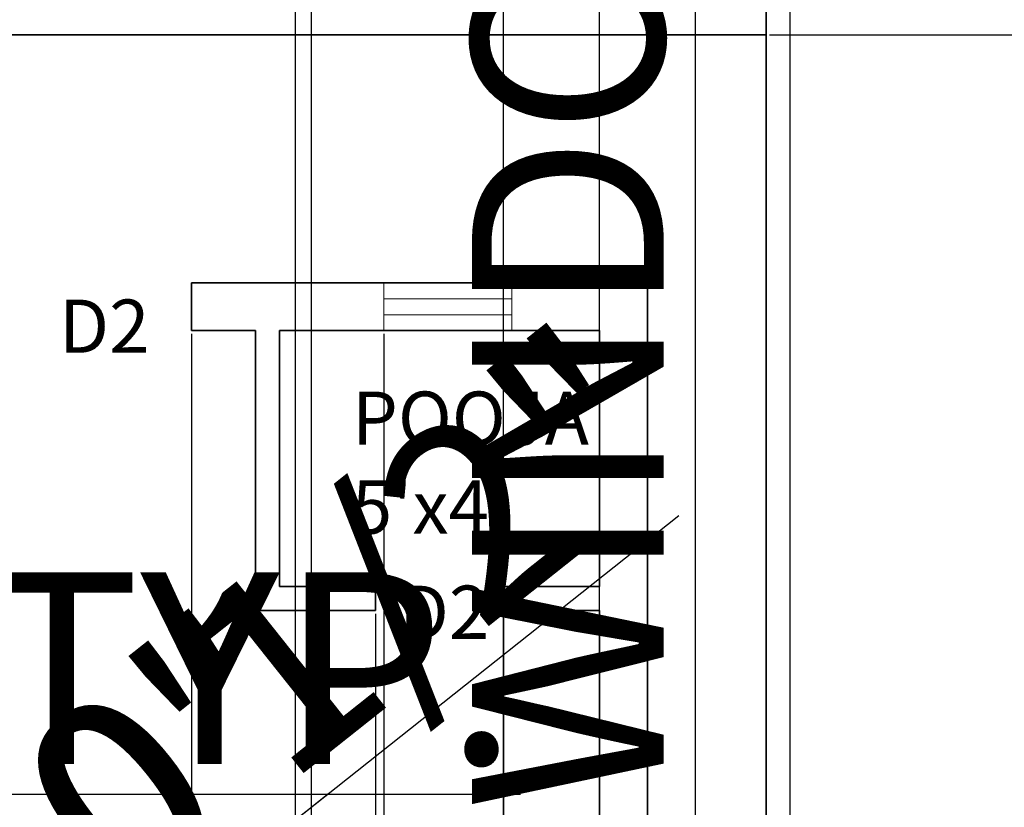
# Model space of a CAD drawing. Units: inches. Extents: x 1041 to 1781, y -140 to 732.
# Tile 4 of 6: x 1359 to 1543, y 358 to 506. Entities that reach past the tile are written whole.
import ezdxf

# ---------------------------------------------------------------- set-up
doc = ezdxf.new("R2010")
doc.units = ezdxf.units.IN
for name, color, linetype, lineweight in [('A-ANNO-TEXT', 7, 'Continuous', 18), ('A-AREA-IDEN', 7, 'Continuous', 20), ('A-GLAZ', 4, 'Continuous', 18), ('A-WALL', 7, 'Continuous', 35), ('C-PROP', 3, 'Continuous', 25), ('dimension', 130, 'Continuous', 18)]:
    doc.layers.add(name, color=color, linetype=linetype, lineweight=lineweight)
doc.styles.get("Standard").update_dxf_attribs({"font": 'arial.ttf'})
doc.dimstyles.new('ISO-25', dxfattribs={"dimtxt": 36, "dimasz": 24, "dimexe": 1.25, "dimexo": 0.625, "dimtad": 1, "dimlunit": 4, "dimtxsty": 'Standard', "dimcen": 2.5, "dimadec": 0, "dimazin": 0, "dimtfac": 1, "dimtmove": 0, "dimatfit": 3, "dimfxl": 1, "dimarcsym": 0})

# ---------------------------------------------------------------- blocks, each defined once
blk = doc.blocks.new('WIN-24IN')
for p, q in [((0, 9), (24, 9)), ((24, 9), (0, 9)), ((0, 9), (0, 0)), ((24, 0), (24, 9)), ((24, 6), (0, 6)), ((0, 3), (24, 3)), ((0, 0), (24, 0))]:
    blk.add_line(p, q)
blk = doc.blocks.new('*D10')
at = {"layer": 'Defpoints', "color": 0, "transparency": 16777216}
for p in [(1174.94, 364.32), (1183.94, 364.32), (1183.94, 360.72)]:
    blk.add_point(p, dxfattribs=at)
at = {"layer": 'dimension', "color": 0, "lineweight": -2, "transparency": 16777216}
for p, q in [((1174.94, 363.69), (1174.94, 359.47)), ((1183.94, 363.69), (1183.94, 359.47)), ((1150.94, 360.72), (1126.94, 360.72)), ((1174.94, 360.72), (1183.94, 360.72)), ((1207.94, 360.72), (1452.63, 360.72))]:
    blk.add_line(p, q, dxfattribs=at)
at = {"layer": 'dimension', "color": 0, "transparency": 16777216}
for points in [[(1150.94, 364.72), (1150.94, 356.72), (1174.94, 360.72)], [(1207.94, 364.72), (1207.94, 356.72), (1183.94, 360.72)]]:
    blk.add_solid(points, dxfattribs=at)
at = {"layer": 'dimension', "color": 0, "transparency": 16777216, "insert": (1342.28, 379.72), "char_height": 36, "attachment_point": 5}
blk.add_mtext('0\'-9" TYP.', dxfattribs=at)
blk = doc.blocks.new('*D13')
at = {"layer": 'Defpoints', "color": 0, "transparency": 16777216}
for p in [(1476.44, 329.99), (1485.44, 329.99), (1476.44, 269.99)]:
    blk.add_point(p, dxfattribs=at)
at = {"layer": 'dimension', "color": 0, "lineweight": -2, "transparency": 16777216}
for p, q in [((1485.44, 329.99), (1485.44, 687.05)), ((1477.06, 329.99), (1486.69, 329.99)), ((1485.44, 293.99), (1485.44, 305.99)), ((1477.06, 269.99), (1486.69, 269.99))]:
    blk.add_line(p, q, dxfattribs=at)
at = {"layer": 'dimension', "color": 0, "transparency": 16777216}
for points in [[(1481.44, 305.99), (1489.44, 305.99), (1485.44, 329.99)], [(1481.44, 293.99), (1489.44, 293.99), (1485.44, 269.99)]]:
    blk.add_solid(points, dxfattribs=at)
at = {"layer": 'dimension', "color": 0, "transparency": 16777216, "insert": (1466.19, 520.52), "char_height": 36, "attachment_point": 5, "rotation": 90}
blk.add_mtext('WINDOW 5\'-0"', dxfattribs=at)
blk = doc.blocks.new('*D16')
at = {"layer": 'Defpoints', "color": 0, "transparency": 16777216}
for p in [(1498.75, 503.23), (1633.79, 503.23), (1498.75, 32.23)]:
    blk.add_point(p, dxfattribs=at)
at = {"layer": 'dimension', "color": 0, "lineweight": -2, "transparency": 16777216}
for p, q in [((1499.37, 503.23), (1635.04, 503.23)), ((1633.79, 56.23), (1633.79, 479.23)), ((1499.37, 32.23), (1635.04, 32.23))]:
    blk.add_line(p, q, dxfattribs=at)
at = {"layer": 'dimension', "color": 0, "transparency": 16777216}
for points in [[(1629.79, 479.23), (1637.79, 479.23), (1633.79, 503.23)], [(1629.79, 56.23), (1637.79, 56.23), (1633.79, 32.23)]]:
    blk.add_solid(points, dxfattribs=at)
at = {"layer": 'dimension', "color": 0, "transparency": 16777216, "insert": (1614.78, 267.73), "char_height": 36, "attachment_point": 5, "rotation": 90}
blk.add_mtext('39\'-3"', dxfattribs=at)
blk = doc.blocks.new('*D18')
at = {"layer": 'Defpoints', "color": 0, "transparency": 16777216}
for p in [(1449.44, 541.68), (1413.44, 207.73), (1449.44, 207.73)]:
    blk.add_point(p, dxfattribs=at)
at = {"layer": 'dimension', "color": 0, "lineweight": -2, "transparency": 16777216}
for p, q in [((1389.44, 541.68), (1365.44, 541.68)), ((1413.44, 208.36), (1413.44, 542.93)), ((1413.44, 541.68), (1449.44, 541.68)), ((1449.44, 208.36), (1449.44, 542.93)), ((1473.44, 541.68), (1594.36, 541.68))]:
    blk.add_line(p, q, dxfattribs=at)
at = {"layer": 'dimension', "color": 0, "transparency": 16777216}
for points in [[(1389.44, 545.68), (1389.44, 537.68), (1413.44, 541.68)], [(1473.44, 545.68), (1473.44, 537.68), (1449.44, 541.68)]]:
    blk.add_solid(points, dxfattribs=at)
at = {"layer": 'dimension', "color": 0, "transparency": 16777216, "insert": (1545.9, 560.7), "char_height": 36, "attachment_point": 5}
blk.add_mtext('3\'-0"', dxfattribs=at)
blk = doc.blocks.new('*D19')
at = {"layer": 'Defpoints', "color": 0, "transparency": 16777216}
for p in [(1354.94, 447.73), (1390.94, 447.73), (1390.94, 2.78)]:
    blk.add_point(p, dxfattribs=at)
at = {"layer": 'dimension', "color": 0, "lineweight": -2, "transparency": 16777216}
for p, q in [((1354.94, 447.11), (1354.94, 1.53)), ((1390.94, 447.11), (1390.94, 1.53)), ((1330.94, 2.78), (1306.94, 2.78)), ((1354.94, 2.78), (1390.94, 2.78)), ((1414.94, 2.78), (1535.86, 2.78))]:
    blk.add_line(p, q, dxfattribs=at)
at = {"layer": 'dimension', "color": 0, "transparency": 16777216}
for points in [[(1330.94, 6.78), (1330.94, -1.22), (1354.94, 2.78)], [(1414.94, 6.78), (1414.94, -1.22), (1390.94, 2.78)]]:
    blk.add_solid(points, dxfattribs=at)
at = {"layer": 'dimension', "color": 0, "transparency": 16777216, "insert": (1487.4, 21.8), "char_height": 36, "attachment_point": 5}
blk.add_mtext('3\'-0"', dxfattribs=at)
blk = doc.blocks.new('*D20')
at = {"layer": 'Defpoints', "color": 0, "transparency": 16777216}
for p in [(1425.44, 395.23), (1449.44, 395.23), (1449.44, 2.78)]:
    blk.add_point(p, dxfattribs=at)
at = {"layer": 'dimension', "color": 0, "lineweight": -2, "transparency": 16777216}
for p, q in [((1425.44, 394.61), (1425.44, 1.53)), ((1449.44, 394.61), (1449.44, 1.53)), ((1401.44, 2.78), (1377.44, 2.78)), ((1425.44, 2.78), (1449.44, 2.78)), ((1473.44, 2.78), (1595, 2.78))]:
    blk.add_line(p, q, dxfattribs=at)
at = {"layer": 'dimension', "color": 0, "transparency": 16777216}
for points in [[(1401.44, 6.78), (1401.44, -1.22), (1425.44, 2.78)], [(1473.44, 6.78), (1473.44, -1.22), (1449.44, 2.78)]]:
    blk.add_solid(points, dxfattribs=at)
at = {"layer": 'dimension', "color": 0, "transparency": 16777216, "insert": (1546.22, 21.79), "char_height": 36, "attachment_point": 5}
blk.add_mtext('2\'-0"', dxfattribs=at)
blk = doc.blocks.new('*D21')
at = {"layer": 'Defpoints', "color": 0, "transparency": 16777216}
for p in [(1449.44, 541.68), (1410.44, 41.23), (1449.44, 41.23)]:
    blk.add_point(p, dxfattribs=at)
at = {"layer": 'dimension', "color": 0, "lineweight": -2, "transparency": 16777216}
for p, q in [((1386.44, 541.68), (1362.44, 541.68)), ((1410.44, 41.86), (1410.44, 542.93)), ((1410.44, 541.68), (1449.44, 541.68)), ((1449.44, 41.86), (1449.44, 542.93)), ((1473.44, 541.68), (1594.36, 541.68))]:
    blk.add_line(p, q, dxfattribs=at)
at = {"layer": 'dimension', "color": 0, "transparency": 16777216}
for points in [[(1386.44, 545.68), (1386.44, 537.68), (1410.44, 541.68)], [(1473.44, 545.68), (1473.44, 537.68), (1449.44, 541.68)]]:
    blk.add_solid(points, dxfattribs=at)
at = {"layer": 'dimension', "color": 0, "transparency": 16777216, "insert": (1545.9, 560.7), "char_height": 36, "attachment_point": 5}
blk.add_mtext('3\'-3"', dxfattribs=at)
blk = doc.blocks.new('*D23')
at = {"layer": 'Defpoints', "color": 0, "transparency": 16777216}
for p in [(1302.68, 270.36), (1321, 247.3), (1302.2, 232.37)]:
    blk.add_point(p, dxfattribs=at)
at = {"layer": 'dimension', "color": 0, "lineweight": -2, "transparency": 16777216}
for p, q in [((1321.47, 285.29), (1416.66, 360.9)), ((1283.89, 255.44), (1302.68, 270.36)), ((1320.61, 247.79), (1301.9, 271.34)), ((1301.82, 232.86), (1283.11, 256.41)), ((1265.09, 240.51), (1246.3, 225.58))]:
    blk.add_line(p, q, dxfattribs=at)
at = {"layer": 'dimension', "color": 0, "transparency": 16777216}
for points in [[(1318.99, 288.42), (1323.96, 282.16), (1302.68, 270.36)], [(1262.61, 243.64), (1267.58, 237.38), (1283.89, 255.44)]]:
    blk.add_solid(points, dxfattribs=at)
at = {"layer": 'dimension', "color": 0, "transparency": 16777216, "insert": (1366.64, 345.44), "char_height": 36, "attachment_point": 5, "rotation": 38.4594}
blk.add_mtext('2\'-0"', dxfattribs=at)
blk = doc.blocks.new('*D29')
at = {"layer": 'Defpoints', "color": 0, "transparency": 16777216}
for p in [(1113.8, 269.99), (1467.44, 269.99), (1467.44, 207.73)]:
    blk.add_point(p, dxfattribs=at)
at = {"layer": 'dimension', "color": 0, "lineweight": -2, "transparency": 16777216}
for p, q in [((1113.8, 269.99), (1113.8, 474.82)), ((1466.81, 269.99), (1112.55, 269.99)), ((1113.8, 231.73), (1113.8, 245.99)), ((1466.81, 207.73), (1112.55, 207.73))]:
    blk.add_line(p, q, dxfattribs=at)
at = {"layer": 'dimension', "color": 0, "transparency": 16777216}
for points in [[(1109.8, 245.99), (1117.8, 245.99), (1113.8, 269.99)], [(1109.8, 231.73), (1117.8, 231.73), (1113.8, 207.73)]]:
    blk.add_solid(points, dxfattribs=at)
at = {"layer": 'dimension', "color": 0, "transparency": 16777216, "insert": (1094.56, 384.41), "char_height": 36, "attachment_point": 5, "rotation": 90}
blk.add_mtext('5\'-2 1/2"', dxfattribs=at)
blk = doc.blocks.new('*D31')
at = {"layer": 'Defpoints', "color": 0, "transparency": 16777216}
for p in [(1390.94, 447.73), (1427, 447.73), (1427, 2.78)]:
    blk.add_point(p, dxfattribs=at)
at = {"layer": 'dimension', "color": 0, "lineweight": -2, "transparency": 16777216}
for p, q in [((1390.94, 447.11), (1390.94, 1.53)), ((1427, 447.11), (1427, 1.53)), ((1366.94, 2.78), (1342.94, 2.78)), ((1390.94, 2.78), (1427, 2.78)), ((1451, 2.78), (1571.93, 2.78))]:
    blk.add_line(p, q, dxfattribs=at)
at = {"layer": 'dimension', "color": 0, "transparency": 16777216}
for points in [[(1366.94, 6.78), (1366.94, -1.22), (1390.94, 2.78)], [(1451, 6.78), (1451, -1.22), (1427, 2.78)]]:
    blk.add_solid(points, dxfattribs=at)
at = {"layer": 'dimension', "color": 0, "transparency": 16777216, "insert": (1523.46, 21.8), "char_height": 36, "attachment_point": 5}
blk.add_mtext('3\'-0"', dxfattribs=at)
blk = doc.blocks.new('*D32')
at = {"layer": 'Defpoints', "color": 0, "transparency": 16777216}
for p in [(1236.44, 447.73), (1278.74, 447.73), (1278.74, 2.78)]:
    blk.add_point(p, dxfattribs=at)
at = {"layer": 'dimension', "color": 0, "lineweight": -2, "transparency": 16777216}
for p, q in [((1236.44, 447.11), (1236.44, 1.53)), ((1278.74, 447.11), (1278.74, 1.53)), ((1212.44, 2.78), (1188.44, 2.78)), ((1236.44, 2.78), (1278.74, 2.78)), ((1302.74, 2.78), (1507.55, 2.78))]:
    blk.add_line(p, q, dxfattribs=at)
at = {"layer": 'dimension', "color": 0, "transparency": 16777216}
for points in [[(1212.44, 6.78), (1212.44, -1.22), (1236.44, 2.78)], [(1302.74, 6.78), (1302.74, -1.22), (1278.74, 2.78)]]:
    blk.add_solid(points, dxfattribs=at)
at = {"layer": 'dimension', "color": 0, "transparency": 16777216, "insert": (1417.15, 22.03), "char_height": 36, "attachment_point": 5}
blk.add_mtext('3\'-6 1/2"', dxfattribs=at)
blk = doc.blocks.new('*D35')
at = {"layer": 'Defpoints', "color": 0, "transparency": 16777216}
for p in [(1321.94, 541.68), (1297.94, 165.73), (1321.94, 165.73)]:
    blk.add_point(p, dxfattribs=at)
at = {"layer": 'dimension', "color": 0, "lineweight": -2, "transparency": 16777216}
for p, q in [((1273.94, 541.68), (1249.94, 541.68)), ((1297.94, 166.36), (1297.94, 542.93)), ((1297.94, 541.68), (1321.94, 541.68)), ((1321.94, 166.36), (1321.94, 542.93)), ((1345.94, 541.68), (1467.5, 541.68))]:
    blk.add_line(p, q, dxfattribs=at)
at = {"layer": 'dimension', "color": 0, "transparency": 16777216}
for points in [[(1273.94, 545.68), (1273.94, 537.68), (1297.94, 541.68)], [(1345.94, 545.68), (1345.94, 537.68), (1321.94, 541.68)]]:
    blk.add_solid(points, dxfattribs=at)
at = {"layer": 'dimension', "color": 0, "transparency": 16777216, "insert": (1418.72, 560.69), "char_height": 36, "attachment_point": 5}
blk.add_mtext('2\'-0"', dxfattribs=at)
blk = doc.blocks.new('*D39')
at = {"layer": 'Defpoints', "color": 0, "transparency": 16777216}
for p in [(1467.44, 541.68), (1449.44, 207.73), (1467.44, 207.73)]:
    blk.add_point(p, dxfattribs=at)
at = {"layer": 'dimension', "color": 0, "lineweight": -2, "transparency": 16777216}
for p, q in [((1425.44, 541.68), (1401.44, 541.68)), ((1449.44, 208.36), (1449.44, 542.93)), ((1449.44, 541.68), (1467.44, 541.68)), ((1467.44, 208.36), (1467.44, 542.93)), ((1491.44, 541.68), (1609, 541.68))]:
    blk.add_line(p, q, dxfattribs=at)
at = {"layer": 'dimension', "color": 0, "transparency": 16777216}
for points in [[(1425.44, 545.68), (1425.44, 537.68), (1449.44, 541.68)], [(1491.44, 545.68), (1491.44, 537.68), (1467.44, 541.68)]]:
    blk.add_solid(points, dxfattribs=at)
at = {"layer": 'dimension', "color": 0, "transparency": 16777216, "insert": (1562.22, 560.69), "char_height": 36, "attachment_point": 5}
blk.add_mtext('1\'-6"', dxfattribs=at)
blk = doc.blocks.new('*D45')
at = {"layer": 'Defpoints', "color": 0, "transparency": 16777216}
for p in [(1283.89, 255.44), (1302.2, 232.37), (1284.4, 218.23)]:
    blk.add_point(p, dxfattribs=at)
at = {"layer": 'dimension', "color": 0, "lineweight": -2, "transparency": 16777216}
for p, q in [((1302.68, 270.36), (1482.32, 413.05)), ((1266.08, 241.29), (1283.89, 255.44)), ((1301.82, 232.86), (1283.11, 256.41)), ((1284.01, 218.72), (1265.3, 242.27)), ((1247.29, 226.37), (1228.5, 211.44))]:
    blk.add_line(p, q, dxfattribs=at)
at = {"layer": 'dimension', "color": 0, "transparency": 16777216}
for points in [[(1300.19, 273.49), (1305.17, 267.23), (1283.89, 255.44)], [(1244.8, 229.5), (1249.78, 223.23), (1266.08, 241.29)]]:
    blk.add_solid(points, dxfattribs=at)
at = {"layer": 'dimension', "color": 0, "transparency": 16777216, "insert": (1389.93, 364.23), "char_height": 36, "attachment_point": 5, "rotation": 38.4594}
blk.add_mtext('1\'-10 1/2"', dxfattribs=at)

msp = doc.modelspace()

# ---------------------------------------------------------------- linework, layer by layer
at = {"layer": 'A-WALL'}
for p, q in [((1498.749, 32.233), (1498.749, 512.233)), ((1498.749, 503.233), (1174.938, 503.233)), ((1390.938, 447.733), (1390.938, 456.733)), ((1390.938, 456.733), (1476.438, 456.733)), ((1476.438, 203.233), (1476.438, 456.733)), ((1390.938, 447.733), (1402.938, 447.733)), ((1402.938, 395.233), (1402.938, 447.733)), ((1407.438, 399.733), (1407.438, 447.733)), ((1407.438, 447.733), (1467.438, 447.733)), ((1467.438, 399.733), (1467.438, 447.733)), ((1407.438, 399.733), (1425.438, 399.733)), ((1425.438, 395.233), (1425.438, 399.733)), ((1449.438, 395.233), (1449.438, 399.733)), ((1449.438, 399.733), (1467.438, 399.733)), ((1402.938, 395.233), (1425.438, 395.233)), ((1449.438, 395.233), (1467.438, 395.233)), ((1467.438, 207.733), (1467.438, 395.233))]:
    msp.add_line(p, q, dxfattribs=at)
at = {"layer": 'C-PROP'}
msp.add_line((1503.249, 32.233), (1503.249, 512.233), dxfattribs=at)

# ---------------------------------------------------------------- block references
at = {"layer": 'A-GLAZ'}
msp.add_blockref('WIN-24IN', (1427.003, 447.733), dxfattribs=at)

# ---------------------------------------------------------------- texts
at = {"layer": 'A-ANNO-TEXT', "char_height": 10, "attachment_point": 1}
for insert in [(1366.081, 453.57), (1429.827, 399.877)]:
    msp.add_mtext_dynamic_manual_height_columns('D2', width=64.5482, gutter_width=12.5, heights=[0], dxfattribs=dict(at, insert=insert))
at = {"layer": 'A-AREA-IDEN', "insert": (1421.004, 436.302), "char_height": 10, "attachment_point": 1}
msp.add_mtext_dynamic_manual_height_columns("POOJA\\P5'x4'", width=64.5482, gutter_width=12.5, heights=[0], dxfattribs=at)

# ---------------------------------------------------------------- dimensions: what is measured, and where the dimension line sits
at = {"layer": 'dimension'}
dim = msp.add_linear_dim(base=(1485.438, 329.99), p1=(1476.438, 269.99), p2=(1476.438, 329.99), angle=90, text='WINDOW <>', dimstyle='ISO-25', override={"dimdec": 1, "dimlfac": 1, "dimrnd": 0, "dimzin": 1, "dimdsep": 46, "dimlunit": 4, "dimfrac": 2}, dxfattribs=at)
dim.commit()
dim.dimension.update_dxf_attribs({"geometry": '*D13', "text_midpoint": (1466.186, 520.519)})
for base, p1, p2, picture, middle in [((1321.938, 541.683), (1297.938, 165.733), (1321.938, 165.733), '*D35', (1418.718, 560.688)), ((1449.438, 541.683), (1410.438, 41.233), (1449.438, 41.233), '*D21', (1545.899, 560.7)), ((1449.438, 541.683), (1413.438, 207.733), (1449.438, 207.733), '*D18', (1545.899, 560.7)), ((1467.438, 541.683), (1449.438, 207.733), (1467.438, 207.733), '*D39', (1562.217, 560.688)), ((1278.743, 2.783), (1236.438, 447.733), (1278.743, 447.733), '*D32', (1417.147, 22.034)), ((1390.938, 2.783), (1354.938, 447.733), (1390.938, 447.733), '*D19', (1487.399, 21.8)), ((1427.003, 2.783), (1390.938, 447.733), (1427.003, 447.733), '*D31', (1523.464, 21.8)), ((1449.438, 2.783), (1425.438, 395.233), (1449.438, 395.233), '*D20', (1546.218, 21.788))]:
    dim = msp.add_linear_dim(base=base, p1=p1, p2=p2, dimstyle='ISO-25', override={"dimdec": 1, "dimlfac": 1, "dimrnd": 0, "dimzin": 1, "dimdsep": 46, "dimlunit": 4, "dimfrac": 2}, dxfattribs=at)
    dim.commit()
    dim.dimension.update_dxf_attribs({"geometry": picture, "text_midpoint": middle})
for base, p1, p2, angle, picture, middle in [((1633.794, 503.233), (1498.749, 32.233), (1498.749, 503.233), 90, '*D16', (1614.777, 267.733)), ((1113.799, 269.99), (1467.438, 207.733), (1467.438, 269.99), 90, '*D29', (1094.56, 384.406)), ((1283.887, 255.436), (1284.399, 218.233), (1302.204, 232.375), 38.45936, '*D45', (1389.932, 364.234)), ((1302.68, 270.363), (1302.204, 232.375), (1320.997, 247.302), 38.45936, '*D23', (1366.644, 345.439))]:
    dim = msp.add_linear_dim(base=base, p1=p1, p2=p2, angle=angle, dimstyle='ISO-25', override={"dimdec": 1, "dimlfac": 1, "dimrnd": 0, "dimzin": 1, "dimdsep": 46, "dimlunit": 4, "dimfrac": 2}, dxfattribs=at)
    dim.commit()
    dim.dimension.update_dxf_attribs({"geometry": picture, "text_midpoint": middle})
dim = msp.add_linear_dim(base=(1183.938, 360.718), p1=(1174.938, 364.318), p2=(1183.938, 364.318), text='<> TYP.', dimstyle='ISO-25', override={"dimdec": 1, "dimlfac": 1, "dimrnd": 0, "dimzin": 1, "dimdsep": 46, "dimlunit": 4, "dimfrac": 2}, dxfattribs=at)
dim.commit()
dim.dimension.update_dxf_attribs({"geometry": '*D10', "text_midpoint": (1342.281, 379.723)})

doc.saveas('drawing.dxf')
